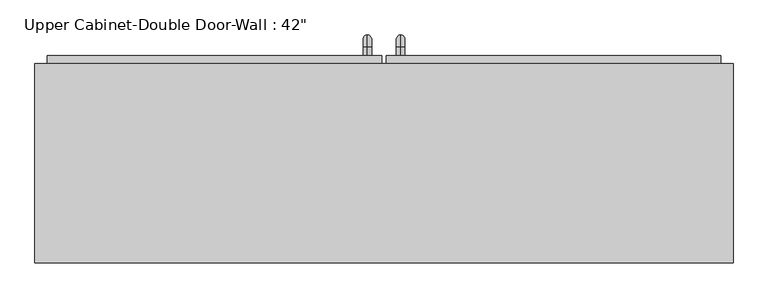
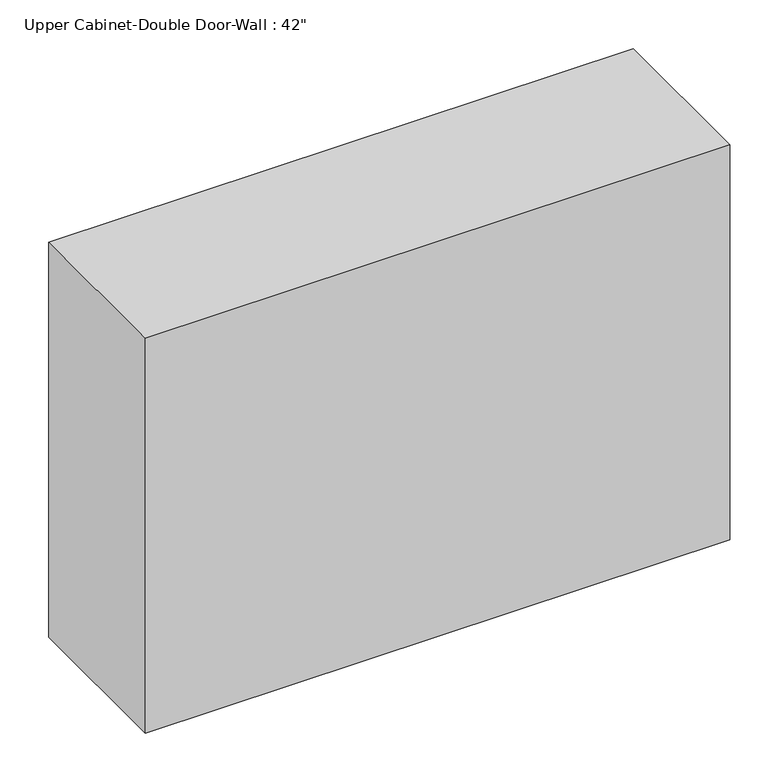
"""IFC4 building model written with IfcOpenShell, lengths in millimetres: furniture geometry."""

from ifc_helpers import new_model, si_unit, point, frame, origin, place, context, project, spatial, polyline, circle_curve, ellipse_curve, trimmed, outline, extrude, faceted_brep, source, transform, mapped, element, save
from ifc_brep_helpers import plane_surface, cylinder_surface, revolved_surface, advanced_brep


def furniture_9929ec1f(model_context):
    return source(origin(), model_context, "Body", "SolidModel", [
        extrude(outline(polyline([(32.9461628, 431.8), (544.1211628, 431.8), (544.1211628, 400.05), (32.9461628, 400.05), (32.9461628, 431.8)])), frame((0.0, 0.0, 1390.65), z_axis=(0.0, 0.0, 1.0), x_axis=(1.0, 0.0, 0.0)), (0.0, 0.0, 1.0), 723.9),
        extrude(outline(polyline([(-484.5788372, 431.8), (26.5961628, 431.8), (26.5961628, 400.05), (-484.5788372, 400.05), (-484.5788372, 431.8)])), frame((0.0, 0.0, 1390.65), z_axis=(0.0, 0.0, 1.0), x_axis=(1.0, 0.0, 0.0)), (0.0, 0.0, 1.0), 723.9),
        advanced_brep(
        [(4.3711628, 431.8, 1517.65), (4.3711628, 431.8, 1530.35), (4.3711628, 444.5, 1517.65), (4.3711628, 444.5, 1530.35), (4.3711628, 463.55, 1511.3), (4.3711628, 450.85, 1511.3), (4.3711628, 450.85, 1435.1), (4.3711628, 463.55, 1435.1), (4.3711628, 444.5, 1416.05), (4.3711628, 444.5, 1428.75), (4.3711628, 431.8, 1428.75), (4.3711628, 431.8, 1416.05)],
        [
            (0, 1, circle_curve(frame((4.3711628, 431.8, 1524.0), z_axis=(0.0, -1.0, 0.0), x_axis=(0.0, 0.0, 1.0)), 6.35)),
            (1, 0, circle_curve(frame((4.3711628, 431.8, 1524.0), z_axis=(0.0, -1.0, 0.0), x_axis=(0.0, 0.0, 1.0)), 6.35)),
            (0, 2),
            (2, 3, circle_curve(frame((4.3711628, 444.5, 1524.0), z_axis=(0.0, -1.0, 0.0), x_axis=(0.0, 0.0, 1.0)), 6.35)),
            (3, 1),
            (3, 2, circle_curve(frame((4.3711628, 444.5, 1524.0), z_axis=(0.0, -1.0, 0.0), x_axis=(0.0, 0.0, 1.0)), 6.35)),
            (4, 3, circle_curve(frame((4.3711628, 444.5, 1511.3), z_axis=(1.0, 0.0, 0.0), x_axis=(0.0, 0.0, 1.0)), 19.05)),
            (2, 5, circle_curve(frame((4.3711628, 444.5, 1511.3), z_axis=(-1.0, 0.0, 0.0), x_axis=(0.0, 0.0, 1.0)), 6.35)),
            (5, 4, circle_curve(frame((4.3711628, 457.2, 1511.3), z_axis=(0.0, 0.0, 1.0), x_axis=(0.0, 1.0, 0.0)), 6.35)),
            (4, 5, circle_curve(frame((4.3711628, 457.2, 1511.3), z_axis=(0.0, 0.0, 1.0), x_axis=(0.0, 1.0, 0.0)), 6.35)),
            (5, 6),
            (6, 7, circle_curve(frame((4.3711628, 457.2, 1435.1), z_axis=(0.0, 0.0, 1.0), x_axis=(0.0, 1.0, 0.0)), 6.35)),
            (7, 4),
            (7, 6, circle_curve(frame((4.3711628, 457.2, 1435.1), z_axis=(0.0, 0.0, 1.0), x_axis=(0.0, 1.0, 0.0)), 6.35)),
            (8, 7, circle_curve(frame((4.3711628, 444.5, 1435.1), z_axis=(1.0, 0.0, 0.0), x_axis=(0.0, 1.0, 0.0)), 19.05)),
            (6, 9, circle_curve(frame((4.3711628, 444.5, 1435.1), z_axis=(-1.0, 0.0, 0.0), x_axis=(0.0, 1.0, 0.0)), 6.35)),
            (9, 8, circle_curve(frame((4.3711628, 444.5, 1422.4), z_axis=(0.0, 1.0, 0.0), x_axis=(0.0, 0.0, -1.0)), 6.35)),
            (8, 9, circle_curve(frame((4.3711628, 444.5, 1422.4), z_axis=(0.0, 1.0, 0.0), x_axis=(0.0, 0.0, -1.0)), 6.35)),
            (10, 11, circle_curve(frame((4.3711628, 431.8, 1422.4), z_axis=(0.0, -1.0, 0.0), x_axis=(0.0, 0.0, -1.0)), 6.35)),
            (11, 10, circle_curve(frame((4.3711628, 431.8, 1422.4), z_axis=(0.0, -1.0, 0.0), x_axis=(0.0, 0.0, -1.0)), 6.35)),
            (9, 10),
            (11, 8),
        ],
        [
            plane_surface(frame((-1.9788372, 431.8, 1524.0), z_axis=(0.0, -1.0, 0.0), x_axis=(0.0, 0.0, 1.0))),
            cylinder_surface(frame((4.3711628, 431.8, 1524.0), z_axis=(0.0, -1.0, 0.0), x_axis=(0.0, 0.0, 1.0)), 6.35),
            revolved_surface(trimmed(ellipse_curve(frame((4.3711628, 444.5, 1524.0), z_axis=(0.0, -1.0, 0.0), x_axis=(0.0, 0.0, 1.0)), 6.35, 6.35), [point((4.3711628, 444.5, 1517.65))], [point((4.3711628, 444.5, 1530.35))], True, "CARTESIAN"), (4.3711628, 444.5, 1511.3), (-1.0, 0.0, 0.0)),
            revolved_surface(trimmed(ellipse_curve(frame((4.3711628, 444.5, 1524.0), z_axis=(0.0, -1.0, 0.0), x_axis=(0.0, 0.0, 1.0)), 6.35, 6.35), [point((4.3711628, 444.5, 1530.35))], [point((4.3711628, 444.5, 1517.65))], True, "CARTESIAN"), (4.3711628, 444.5, 1511.3), (-1.0, 0.0, 0.0)),
            cylinder_surface(frame((4.3711628, 457.2, 1511.3), z_axis=(0.0, 0.0, 1.0), x_axis=(0.0, 1.0, 0.0)), 6.35),
            revolved_surface(trimmed(ellipse_curve(frame((4.3711628, 457.2, 1435.1), z_axis=(0.0, 0.0, 1.0), x_axis=(0.0, 1.0, 0.0)), 6.35, 6.35), [point((4.3711628, 450.85, 1435.1))], [point((4.3711628, 463.55, 1435.1))], True, "CARTESIAN"), (4.3711628, 444.5, 1435.1), (-1.0, 0.0, 0.0)),
            revolved_surface(trimmed(ellipse_curve(frame((4.3711628, 457.2, 1435.1), z_axis=(0.0, 0.0, 1.0), x_axis=(0.0, 1.0, 0.0)), 6.35, 6.35), [point((4.3711628, 463.55, 1435.1))], [point((4.3711628, 450.85, 1435.1))], True, "CARTESIAN"), (4.3711628, 444.5, 1435.1), (-1.0, 0.0, 0.0)),
            plane_surface(frame((-1.9788372, 431.8, 1422.4), z_axis=(0.0, -1.0, 0.0), x_axis=(0.0, 0.0, -1.0))),
            cylinder_surface(frame((4.3711628, 444.5, 1422.4), z_axis=(0.0, 1.0, 0.0), x_axis=(0.0, 0.0, -1.0)), 6.35),
        ],
        [
            (0, [[1, 2]]),
            (1, [[-1, 3, 4, 5]]),
            (1, [[-2, -5, 6, -3]]),
            (2, [[7, -4, 8, 9]]),
            (3, [[-8, -6, -7, 10]]),
            (4, [[-9, 11, 12, 13]]),
            (4, [[-10, -13, 14, -11]]),
            (5, [[15, -12, 16, 17]]),
            (6, [[-16, -14, -15, 18]]),
            (7, [[19, 20]]),
            (8, [[-17, 21, -20, 22]]),
            (8, [[-18, -22, -19, -21]]),
        ],
    ),
        advanced_brep(
        [(55.1711628, 431.8, 1517.65), (55.1711628, 431.8, 1530.35), (55.1711628, 444.5, 1517.65), (55.1711628, 444.5, 1530.35), (55.1711628, 463.55, 1511.3), (55.1711628, 450.85, 1511.3), (55.1711628, 450.85, 1435.1), (55.1711628, 463.55, 1435.1), (55.1711628, 444.5, 1416.05), (55.1711628, 444.5, 1428.75), (55.1711628, 431.8, 1428.75), (55.1711628, 431.8, 1416.05)],
        [
            (0, 1, circle_curve(frame((55.1711628, 431.8, 1524.0), z_axis=(0.0, -1.0, 0.0), x_axis=(0.0, 0.0, -1.0)), 6.35)),
            (1, 0, circle_curve(frame((55.1711628, 431.8, 1524.0), z_axis=(0.0, -1.0, 0.0), x_axis=(0.0, 0.0, -1.0)), 6.35)),
            (0, 2),
            (2, 3, circle_curve(frame((55.1711628, 444.5, 1524.0), z_axis=(0.0, -1.0, 0.0), x_axis=(0.0, 0.0, -1.0)), 6.35)),
            (3, 1),
            (3, 2, circle_curve(frame((55.1711628, 444.5, 1524.0), z_axis=(0.0, -1.0, 0.0), x_axis=(0.0, 0.0, -1.0)), 6.35)),
            (4, 3, circle_curve(frame((55.1711628, 444.5, 1511.3), z_axis=(1.0, 0.0, 0.0), x_axis=(0.0, 0.0, 1.0)), 19.05)),
            (2, 5, circle_curve(frame((55.1711628, 444.5, 1511.3), z_axis=(-1.0, 0.0, 0.0), x_axis=(0.0, 0.0, 1.0)), 6.35)),
            (5, 4, circle_curve(frame((55.1711628, 457.2, 1511.3), z_axis=(0.0, 0.0, 1.0), x_axis=(0.0, -1.0, 0.0)), 6.35)),
            (4, 5, circle_curve(frame((55.1711628, 457.2, 1511.3), z_axis=(0.0, 0.0, 1.0), x_axis=(0.0, -1.0, 0.0)), 6.35)),
            (5, 6),
            (6, 7, circle_curve(frame((55.1711628, 457.2, 1435.1), z_axis=(0.0, 0.0, 1.0), x_axis=(0.0, -1.0, 0.0)), 6.35)),
            (7, 4),
            (7, 6, circle_curve(frame((55.1711628, 457.2, 1435.1), z_axis=(0.0, 0.0, 1.0), x_axis=(0.0, -1.0, 0.0)), 6.35)),
            (8, 7, circle_curve(frame((55.1711628, 444.5, 1435.1), z_axis=(1.0, 0.0, 0.0), x_axis=(0.0, 1.0, 0.0)), 19.05)),
            (6, 9, circle_curve(frame((55.1711628, 444.5, 1435.1), z_axis=(-1.0, 0.0, 0.0), x_axis=(0.0, 1.0, 0.0)), 6.35)),
            (9, 8, circle_curve(frame((55.1711628, 444.5, 1422.4), z_axis=(0.0, 1.0, 0.0), x_axis=(0.0, 0.0, 1.0)), 6.35)),
            (8, 9, circle_curve(frame((55.1711628, 444.5, 1422.4), z_axis=(0.0, 1.0, 0.0), x_axis=(0.0, 0.0, 1.0)), 6.35)),
            (10, 11, circle_curve(frame((55.1711628, 431.8, 1422.4), z_axis=(0.0, -1.0, 0.0), x_axis=(0.0, 0.0, 1.0)), 6.35)),
            (11, 10, circle_curve(frame((55.1711628, 431.8, 1422.4), z_axis=(0.0, -1.0, 0.0), x_axis=(0.0, 0.0, 1.0)), 6.35)),
            (9, 10),
            (11, 8),
        ],
        [
            plane_surface(frame((48.8211628, 431.8, 1524.0), z_axis=(0.0, -1.0, 0.0), x_axis=(0.0, 0.0, 1.0))),
            cylinder_surface(frame((55.1711628, 431.8, 1524.0), z_axis=(0.0, -1.0, 0.0), x_axis=(0.0, 0.0, -1.0)), 6.35),
            revolved_surface(trimmed(ellipse_curve(frame((55.1711628, 444.5, 1524.0), z_axis=(0.0, -1.0, 0.0), x_axis=(0.0, 0.0, -1.0)), 6.35, 6.35), [point((55.1711628, 444.5, 1517.65))], [point((55.1711628, 444.5, 1530.35))], True, "CARTESIAN"), (55.1711628, 444.5, 1511.3), (-1.0, 0.0, 0.0)),
            revolved_surface(trimmed(ellipse_curve(frame((55.1711628, 444.5, 1524.0), z_axis=(0.0, -1.0, 0.0), x_axis=(0.0, 0.0, -1.0)), 6.35, 6.35), [point((55.1711628, 444.5, 1530.35))], [point((55.1711628, 444.5, 1517.65))], True, "CARTESIAN"), (55.1711628, 444.5, 1511.3), (-1.0, 0.0, 0.0)),
            cylinder_surface(frame((55.1711628, 457.2, 1511.3), z_axis=(0.0, 0.0, 1.0), x_axis=(0.0, -1.0, 0.0)), 6.35),
            revolved_surface(trimmed(ellipse_curve(frame((55.1711628, 457.2, 1435.1), z_axis=(0.0, 0.0, 1.0), x_axis=(0.0, -1.0, 0.0)), 6.35, 6.35), [point((55.1711628, 450.85, 1435.1))], [point((55.1711628, 463.55, 1435.1))], True, "CARTESIAN"), (55.1711628, 444.5, 1435.1), (-1.0, 0.0, 0.0)),
            revolved_surface(trimmed(ellipse_curve(frame((55.1711628, 457.2, 1435.1), z_axis=(0.0, 0.0, 1.0), x_axis=(0.0, -1.0, 0.0)), 6.35, 6.35), [point((55.1711628, 463.55, 1435.1))], [point((55.1711628, 450.85, 1435.1))], True, "CARTESIAN"), (55.1711628, 444.5, 1435.1), (-1.0, 0.0, 0.0)),
            plane_surface(frame((48.8211628, 431.8, 1422.4), z_axis=(0.0, -1.0, 0.0), x_axis=(0.0, 0.0, -1.0))),
            cylinder_surface(frame((55.1711628, 444.5, 1422.4), z_axis=(0.0, 1.0, 0.0), x_axis=(0.0, 0.0, 1.0)), 6.35),
        ],
        [
            (0, [[1, 2]]),
            (1, [[-1, 3, 4, 5]]),
            (1, [[-2, -5, 6, -3]]),
            (2, [[7, -4, 8, 9]]),
            (3, [[-8, -6, -7, 10]]),
            (4, [[-9, 11, 12, 13]]),
            (4, [[-10, -13, 14, -11]]),
            (5, [[15, -12, 16, 17]]),
            (6, [[-16, -14, -15, 18]]),
            (7, [[19, 20]]),
            (8, [[-17, 21, -20, 22]]),
            (8, [[-18, -22, -19, -21]]),
        ],
    ),
        faceted_brep([(-503.6288372, 114.3, 2133.6), (-503.6288372, 114.3, 1371.6), (563.1711628, 114.3, 1371.6), (563.1711628, 114.3, 2133.6), (-503.6288372, 419.1, 2133.6), (563.1711628, 419.1, 2133.6), (563.1711628, 419.1, 1371.6), (-503.6288372, 419.1, 1371.6), (-484.5788372, 419.1, 2114.55), (-484.5788372, 419.1, 1390.65), (544.1211628, 419.1, 1390.65), (544.1211628, 419.1, 2114.55), (544.1211628, 133.35, 2114.55), (-484.5788372, 133.35, 2114.55), (544.1211628, 133.35, 1390.65), (-484.5788372, 133.35, 1390.65)], [[[0, 1, 2, 3]], [[4, 5, 6, 7], [8, 9, 10, 11]], [[1, 0, 4, 7]], [[2, 1, 7, 6]], [[3, 2, 6, 5]], [[0, 3, 5, 4]], [[8, 11, 12, 13]], [[11, 10, 14, 12]], [[10, 9, 15, 14]], [[9, 8, 13, 15]], [[13, 12, 14, 15]]]),
    ])


if __name__ == "__main__":
    model = new_model("IFC4")
    model_context = context("Model", 3, world=origin())
    ifc_project = project(units=[si_unit("LENGTHUNIT", "METRE", prefix="MILLI")], contexts=[model_context])
    site = spatial("IfcSite", under=ifc_project)
    building = spatial("IfcBuilding", under=site)
    placement = place(None, origin())
    furniture_shape = furniture_9929ec1f(model_context)
    element("IfcFurniture", 1, ObjectType="Upper Cabinet-Double Door-Wall : 42\"", at=placement, inside=building, context=model_context, shape_type="MappedRepresentation", body=[
        mapped(furniture_shape, transform((0.0, 0.0, 0.0), x_axis=(1.0, 0.0, 0.0), y_axis=(0.0, 1.0, 0.0), z_axis=(0.0, 0.0, 1.0))),
    ])
    save(model, "model.ifc")

# Revit data of these elements
# Type "Upper Cabinet-Double Door-Wall : 42\""
#   Assembly Code = "C1030410"
#   Depth = 1' - 0"
#   Height = 2' - 6"
#   Top Of Cabinet = 7' - 0"
#   Width = 3' - 6"
#   Cabinet Material = none
#   Door/Drawer Material = none
#   Handle Material = Cabinets - Handles
#   Default Elevation = 0
# Element 1 (IfcFurniture, "Upper Cabinet-Double Door-Wall : 42\"")
#   Materials on its faces: "Cabinets - Handles", "Cabinet"
# Materials
#   "Cabinets - Handles": colour RGB 57 57 57, transparency 0
#   "Cabinet": colour RGB 204 122 2, transparency 0
